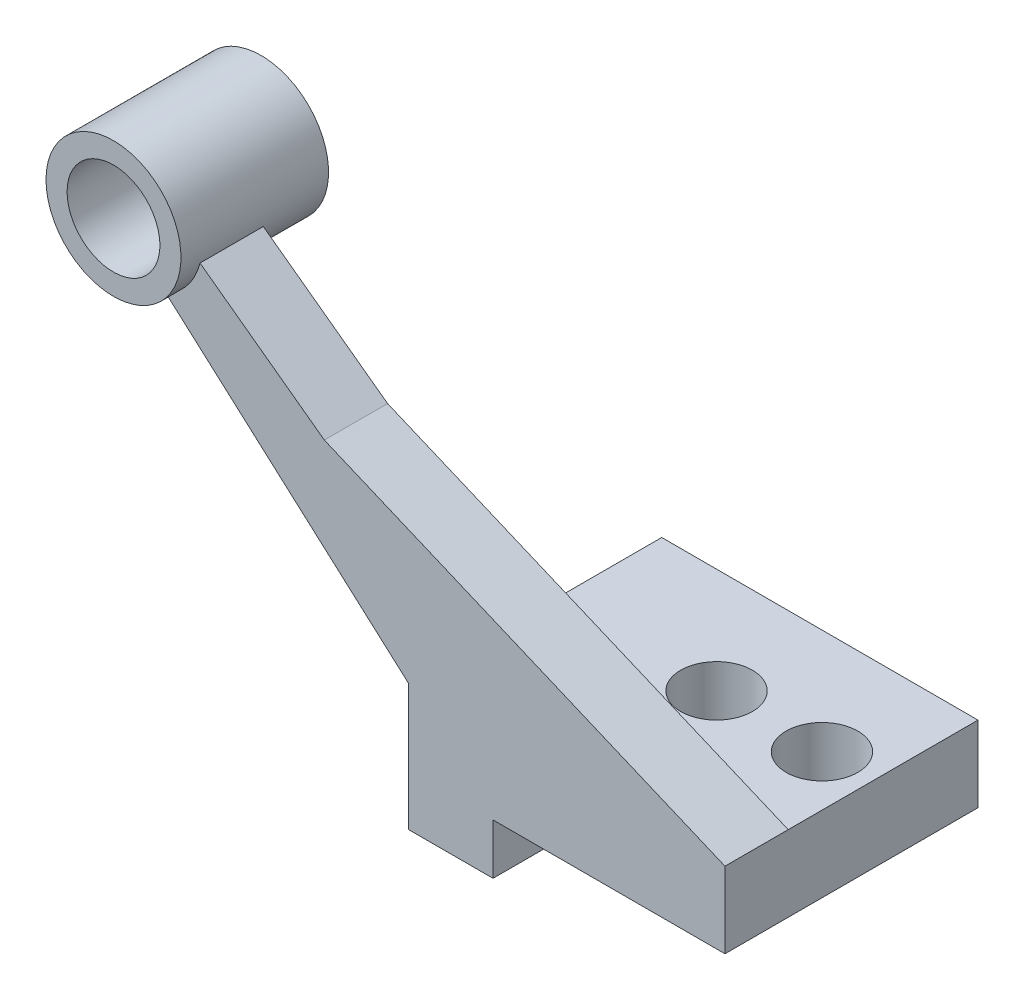
ISO-10303-21;
HEADER;
FILE_DESCRIPTION(('STEP AP214'),'2;1');
FILE_NAME('part.step','',(''),(''),'','','');
FILE_SCHEMA(('AUTOMOTIVE_DESIGN { 1 0 10303 214 1 1 1 1 }'));
ENDSEC;
DATA;
#1=APPLICATION_CONTEXT('core data for automotive mechanical design processes');
#2=APPLICATION_PROTOCOL_DEFINITION('international standard','automotive_design',2000,#1);
#3=PRODUCT_CONTEXT('',#1,'mechanical');
#4=PRODUCT('Part','Part','',(#3));
#5=PRODUCT_RELATED_PRODUCT_CATEGORY('part','',(#4));
#6=PRODUCT_DEFINITION_FORMATION('','',#4);
#7=PRODUCT_DEFINITION_CONTEXT('part definition',#1,'design');
#8=PRODUCT_DEFINITION('design','',#6,#7);
#9=PRODUCT_DEFINITION_SHAPE('','',#8);
#10=(LENGTH_UNIT() NAMED_UNIT(*) SI_UNIT(.MILLI.,.METRE.));
#11=(NAMED_UNIT(*) PLANE_ANGLE_UNIT() SI_UNIT($,.RADIAN.));
#12=(NAMED_UNIT(*) SI_UNIT($,.STERADIAN.) SOLID_ANGLE_UNIT());
#13=UNCERTAINTY_MEASURE_WITH_UNIT(LENGTH_MEASURE(1.E-05),#10,'distance_accuracy_value','');
#14=(GEOMETRIC_REPRESENTATION_CONTEXT(3) GLOBAL_UNCERTAINTY_ASSIGNED_CONTEXT((#13)) GLOBAL_UNIT_ASSIGNED_CONTEXT((#10,
#11,#12)) REPRESENTATION_CONTEXT('',''));
#15=CARTESIAN_POINT('',(0.,0.,0.));
#16=DIRECTION('',(0.,0.,1.));
#17=DIRECTION('',(1.,0.,0.));
#18=AXIS2_PLACEMENT_3D('',#15,#16,#17);
#19=CARTESIAN_POINT('',(0.,0.,45.));
#20=DIRECTION('',(0.,0.,-1.));
#21=DIRECTION('',(-1.,0.,0.));
#22=AXIS2_PLACEMENT_3D('',#19,#20,#21);
#23=PLANE('',#22);
#24=DIRECTION('',(-0.746141301283538,0.665787622683772,0.));
#25=VECTOR('',#24,1.);
#26=CARTESIAN_POINT('',(-140.,58.,45.));
#27=LINE('',#26,#25);
#28=CARTESIAN_POINT('',(-75.,0.,45.));
#29=VERTEX_POINT('',#28);
#30=CARTESIAN_POINT('',(-132.541527054624,51.3447472179725,45.));
#31=VERTEX_POINT('',#30);
#32=EDGE_CURVE('E145',#29,#31,#27,.T.);
#33=ORIENTED_EDGE('',*,*,#32,.T.);
#34=CARTESIAN_POINT('',(-140.,65.5,45.));
#35=DIRECTION('',(0.,0.,-1.));
#36=DIRECTION('',(-1.,0.,0.));
#37=AXIS2_PLACEMENT_3D('',#34,#35,#36);
#38=CIRCLE('',#37,16.);
#39=CARTESIAN_POINT('',(-124.478234627449,61.617372060129,45.));
#40=VERTEX_POINT('',#39);
#41=EDGE_CURVE('E126',#40,#31,#38,.T.);
#42=ORIENTED_EDGE('',*,*,#41,.F.);
#43=DIRECTION('',(0.806404995855705,-0.591363663627518,0.));
#44=VECTOR('',#43,1.);
#45=CARTESIAN_POINT('',(-95.,40.,45.));
#46=LINE('',#45,#44);
#47=CARTESIAN_POINT('',(-95.,40.,45.));
#48=VERTEX_POINT('',#47);
#49=EDGE_CURVE('E133',#40,#48,#46,.T.);
#50=ORIENTED_EDGE('',*,*,#49,.T.);
#51=DIRECTION('',(0.921635375138065,-0.388057000058133,0.));
#52=VECTOR('',#51,1.);
#53=CARTESIAN_POINT('',(0.,0.,45.));
#54=LINE('',#53,#52);
#55=CARTESIAN_POINT('',(0.,0.,45.));
#56=VERTEX_POINT('',#55);
#57=EDGE_CURVE('E142',#48,#56,#54,.T.);
#58=ORIENTED_EDGE('',*,*,#57,.T.);
#59=DIRECTION('',(-1.,0.,0.));
#60=VECTOR('',#59,1.);
#61=CARTESIAN_POINT('',(-75.,0.,45.));
#62=LINE('',#61,#60);
#63=EDGE_CURVE('E159',#56,#29,#62,.T.);
#64=ORIENTED_EDGE('',*,*,#63,.T.);
#65=EDGE_LOOP('',(#33,#42,#50,#58,#64));
#66=FACE_BOUND('',#65,.T.);
#67=ADVANCED_FACE('F44',(#66),#23,.T.);
#68=CARTESIAN_POINT('',(-140.,73.,60.));
#69=DIRECTION('',(0.591363663627518,0.806404995855705,0.));
#70=DIRECTION('',(-0.806404995855705,0.591363663627518,0.));
#71=AXIS2_PLACEMENT_3D('',#68,#69,#70);
#72=PLANE('',#71);
#73=DIRECTION('',(0.,0.,-1.));
#74=VECTOR('',#73,1.);
#75=CARTESIAN_POINT('',(-124.478234627449,61.617372060129,65.));
#76=LINE('',#75,#74);
#77=CARTESIAN_POINT('',(-124.478234627449,61.617372060129,60.));
#78=VERTEX_POINT('',#77);
#79=EDGE_CURVE('E121',#78,#40,#76,.T.);
#80=ORIENTED_EDGE('',*,*,#79,.F.);
#81=DIRECTION('',(0.806404995855705,-0.591363663627518,0.));
#82=VECTOR('',#81,1.);
#83=CARTESIAN_POINT('',(-140.,73.,60.));
#84=LINE('',#83,#82);
#85=CARTESIAN_POINT('',(-95.,40.,60.));
#86=VERTEX_POINT('',#85);
#87=EDGE_CURVE('E170',#78,#86,#84,.T.);
#88=ORIENTED_EDGE('',*,*,#87,.T.);
#89=DIRECTION('',(0.,0.,-1.));
#90=VECTOR('',#89,1.);
#91=CARTESIAN_POINT('',(-95.,40.,60.));
#92=LINE('',#91,#90);
#93=EDGE_CURVE('E140',#86,#48,#92,.T.);
#94=ORIENTED_EDGE('',*,*,#93,.T.);
#95=ORIENTED_EDGE('',*,*,#49,.F.);
#96=EDGE_LOOP('',(#80,#88,#94,#95));
#97=FACE_BOUND('',#96,.T.);
#98=ADVANCED_FACE('F135',(#97),#72,.T.);
#99=CARTESIAN_POINT('',(-75.,0.,60.));
#100=DIRECTION('',(-0.665787622683772,-0.746141301283538,0.));
#101=DIRECTION('',(0.746141301283538,-0.665787622683772,0.));
#102=AXIS2_PLACEMENT_3D('',#99,#100,#101);
#103=PLANE('',#102);
#104=DIRECTION('',(0.,0.,-1.));
#105=VECTOR('',#104,1.);
#106=CARTESIAN_POINT('',(-132.541527054624,51.3447472179725,65.));
#107=LINE('',#106,#105);
#108=CARTESIAN_POINT('',(-132.541527054624,51.3447472179725,60.));
#109=VERTEX_POINT('',#108);
#110=EDGE_CURVE('E67',#31,#109,#107,.F.);
#111=ORIENTED_EDGE('',*,*,#110,.F.);
#112=ORIENTED_EDGE('',*,*,#32,.F.);
#113=DIRECTION('',(0.,0.,-1.));
#114=VECTOR('',#113,1.);
#115=CARTESIAN_POINT('',(-75.,0.,60.));
#116=LINE('',#115,#114);
#117=CARTESIAN_POINT('',(-75.,0.,60.));
#118=VERTEX_POINT('',#117);
#119=EDGE_CURVE('E52',#118,#29,#116,.T.);
#120=ORIENTED_EDGE('',*,*,#119,.F.);
#121=DIRECTION('',(-0.746141301283538,0.665787622683772,0.));
#122=VECTOR('',#121,1.);
#123=CARTESIAN_POINT('',(-75.,0.,60.));
#124=LINE('',#123,#122);
#125=EDGE_CURVE('E172',#118,#109,#124,.T.);
#126=ORIENTED_EDGE('',*,*,#125,.T.);
#127=EDGE_LOOP('',(#111,#112,#120,#126));
#128=FACE_BOUND('',#127,.T.);
#129=ADVANCED_FACE('F213',(#128),#103,.T.);
#130=CARTESIAN_POINT('',(0.,0.,60.));
#131=DIRECTION('',(0.388057000058133,0.921635375138065,0.));
#132=DIRECTION('',(-0.921635375138065,0.388057000058133,0.));
#133=AXIS2_PLACEMENT_3D('',#130,#131,#132);
#134=PLANE('',#133);
#135=DIRECTION('',(0.,0.,-1.));
#136=VECTOR('',#135,1.);
#137=CARTESIAN_POINT('',(0.,0.,60.));
#138=LINE('',#137,#136);
#139=CARTESIAN_POINT('',(0.,0.,60.));
#140=VERTEX_POINT('',#139);
#141=EDGE_CURVE('E11',#140,#56,#138,.T.);
#142=ORIENTED_EDGE('',*,*,#141,.T.);
#143=ORIENTED_EDGE('',*,*,#57,.F.);
#144=ORIENTED_EDGE('',*,*,#93,.F.);
#145=DIRECTION('',(0.921635375138065,-0.388057000058133,0.));
#146=VECTOR('',#145,1.);
#147=CARTESIAN_POINT('',(0.,0.,60.));
#148=LINE('',#147,#146);
#149=EDGE_CURVE('E171',#86,#140,#148,.T.);
#150=ORIENTED_EDGE('',*,*,#149,.T.);
#151=EDGE_LOOP('',(#142,#143,#144,#150));
#152=FACE_BOUND('',#151,.T.);
#153=ADVANCED_FACE('F237',(#152),#134,.T.);
#154=CARTESIAN_POINT('',(0.,-18.,60.));
#155=DIRECTION('',(-1.,0.,0.));
#156=DIRECTION('',(0.,0.,1.));
#157=AXIS2_PLACEMENT_3D('',#154,#155,#156);
#158=PLANE('',#157);
#159=DIRECTION('',(0.,1.,0.));
#160=VECTOR('',#159,1.);
#161=CARTESIAN_POINT('',(0.,-18.,0.));
#162=LINE('',#161,#160);
#163=CARTESIAN_POINT('',(0.,-18.,0.));
#164=VERTEX_POINT('',#163);
#165=CARTESIAN_POINT('',(0.,0.,0.));
#166=VERTEX_POINT('',#165);
#167=EDGE_CURVE('E180',#164,#166,#162,.T.);
#168=ORIENTED_EDGE('',*,*,#167,.T.);
#169=DIRECTION('',(0.,0.,-1.));
#170=VECTOR('',#169,1.);
#171=CARTESIAN_POINT('',(0.,0.,45.));
#172=LINE('',#171,#170);
#173=EDGE_CURVE('E164',#56,#166,#172,.T.);
#174=ORIENTED_EDGE('',*,*,#173,.F.);
#175=ORIENTED_EDGE('',*,*,#141,.F.);
#176=DIRECTION('',(0.,1.,0.));
#177=VECTOR('',#176,1.);
#178=CARTESIAN_POINT('',(0.,-18.,60.));
#179=LINE('',#178,#177);
#180=CARTESIAN_POINT('',(0.,-18.,60.));
#181=VERTEX_POINT('',#180);
#182=EDGE_CURVE('E178',#181,#140,#179,.T.);
#183=ORIENTED_EDGE('',*,*,#182,.F.);
#184=DIRECTION('',(0.,0.,-1.));
#185=VECTOR('',#184,1.);
#186=CARTESIAN_POINT('',(0.,-18.,60.));
#187=LINE('',#186,#185);
#188=EDGE_CURVE('E186',#181,#164,#187,.T.);
#189=ORIENTED_EDGE('',*,*,#188,.T.);
#190=EDGE_LOOP('',(#168,#174,#175,#183,#189));
#191=FACE_BOUND('',#190,.T.);
#192=ADVANCED_FACE('F50',(#191),#158,.F.);
#193=CARTESIAN_POINT('',(-75.,0.,60.));
#194=DIRECTION('',(1.,0.,0.));
#195=DIRECTION('',(0.,0.,-1.));
#196=AXIS2_PLACEMENT_3D('',#193,#194,#195);
#197=PLANE('',#196);
#198=DIRECTION('',(0.,-1.,0.));
#199=VECTOR('',#198,1.);
#200=CARTESIAN_POINT('',(-75.,0.,0.));
#201=LINE('',#200,#199);
#202=CARTESIAN_POINT('',(-75.,0.,0.));
#203=VERTEX_POINT('',#202);
#204=CARTESIAN_POINT('',(-75.,-30.,0.));
#205=VERTEX_POINT('',#204);
#206=EDGE_CURVE('E195',#203,#205,#201,.T.);
#207=ORIENTED_EDGE('',*,*,#206,.T.);
#208=DIRECTION('',(0.,0.,-1.));
#209=VECTOR('',#208,1.);
#210=CARTESIAN_POINT('',(-75.,-30.,60.));
#211=LINE('',#210,#209);
#212=CARTESIAN_POINT('',(-75.,-30.,60.));
#213=VERTEX_POINT('',#212);
#214=EDGE_CURVE('E210',#213,#205,#211,.T.);
#215=ORIENTED_EDGE('',*,*,#214,.F.);
#216=DIRECTION('',(0.,-1.,0.));
#217=VECTOR('',#216,1.);
#218=CARTESIAN_POINT('',(-75.,0.,60.));
#219=LINE('',#218,#217);
#220=EDGE_CURVE('E179',#118,#213,#219,.T.);
#221=ORIENTED_EDGE('',*,*,#220,.F.);
#222=ORIENTED_EDGE('',*,*,#119,.T.);
#223=DIRECTION('',(0.,0.,-1.));
#224=VECTOR('',#223,1.);
#225=CARTESIAN_POINT('',(-75.,0.,45.));
#226=LINE('',#225,#224);
#227=EDGE_CURVE('E161',#29,#203,#226,.T.);
#228=ORIENTED_EDGE('',*,*,#227,.T.);
#229=EDGE_LOOP('',(#207,#215,#221,#222,#228));
#230=FACE_BOUND('',#229,.T.);
#231=ADVANCED_FACE('F215',(#230),#197,.F.);
#232=CARTESIAN_POINT('',(-75.,-30.,60.));
#233=DIRECTION('',(0.,1.,0.));
#234=DIRECTION('',(0.,0.,1.));
#235=AXIS2_PLACEMENT_3D('',#232,#233,#234);
#236=PLANE('',#235);
#237=DIRECTION('',(1.,0.,0.));
#238=VECTOR('',#237,1.);
#239=CARTESIAN_POINT('',(-75.,-30.,0.));
#240=LINE('',#239,#238);
#241=CARTESIAN_POINT('',(-55.,-30.,0.));
#242=VERTEX_POINT('',#241);
#243=EDGE_CURVE('E191',#205,#242,#240,.T.);
#244=ORIENTED_EDGE('',*,*,#243,.T.);
#245=DIRECTION('',(0.,0.,-1.));
#246=VECTOR('',#245,1.);
#247=CARTESIAN_POINT('',(-55.,-30.,60.));
#248=LINE('',#247,#246);
#249=CARTESIAN_POINT('',(-55.,-30.,60.));
#250=VERTEX_POINT('',#249);
#251=EDGE_CURVE('E204',#250,#242,#248,.T.);
#252=ORIENTED_EDGE('',*,*,#251,.F.);
#253=DIRECTION('',(1.,0.,0.));
#254=VECTOR('',#253,1.);
#255=CARTESIAN_POINT('',(-75.,-30.,60.));
#256=LINE('',#255,#254);
#257=EDGE_CURVE('E182',#213,#250,#256,.T.);
#258=ORIENTED_EDGE('',*,*,#257,.F.);
#259=ORIENTED_EDGE('',*,*,#214,.T.);
#260=EDGE_LOOP('',(#244,#252,#258,#259));
#261=FACE_BOUND('',#260,.T.);
#262=ADVANCED_FACE('F223',(#261),#236,.F.);
#263=CARTESIAN_POINT('',(-55.,-30.,60.));
#264=DIRECTION('',(-1.,0.,0.));
#265=DIRECTION('',(0.,0.,1.));
#266=AXIS2_PLACEMENT_3D('',#263,#264,#265);
#267=PLANE('',#266);
#268=DIRECTION('',(0.,1.,0.));
#269=VECTOR('',#268,1.);
#270=CARTESIAN_POINT('',(-55.,-30.,0.));
#271=LINE('',#270,#269);
#272=CARTESIAN_POINT('',(-55.,-18.,0.));
#273=VERTEX_POINT('',#272);
#274=EDGE_CURVE('E196',#242,#273,#271,.T.);
#275=ORIENTED_EDGE('',*,*,#274,.T.);
#276=DIRECTION('',(0.,0.,-1.));
#277=VECTOR('',#276,1.);
#278=CARTESIAN_POINT('',(-55.,-18.,60.));
#279=LINE('',#278,#277);
#280=CARTESIAN_POINT('',(-55.,-18.,60.));
#281=VERTEX_POINT('',#280);
#282=EDGE_CURVE('E203',#281,#273,#279,.T.);
#283=ORIENTED_EDGE('',*,*,#282,.F.);
#284=DIRECTION('',(0.,1.,0.));
#285=VECTOR('',#284,1.);
#286=CARTESIAN_POINT('',(-55.,-30.,60.));
#287=LINE('',#286,#285);
#288=EDGE_CURVE('E184',#250,#281,#287,.T.);
#289=ORIENTED_EDGE('',*,*,#288,.F.);
#290=ORIENTED_EDGE('',*,*,#251,.T.);
#291=EDGE_LOOP('',(#275,#283,#289,#290));
#292=FACE_BOUND('',#291,.T.);
#293=ADVANCED_FACE('F228',(#292),#267,.F.);
#294=CARTESIAN_POINT('',(-55.,-18.,60.));
#295=DIRECTION('',(0.,1.,0.));
#296=DIRECTION('',(0.,0.,1.));
#297=AXIS2_PLACEMENT_3D('',#294,#295,#296);
#298=PLANE('',#297);
#299=CARTESIAN_POINT('',(-12.,-18.,25.));
#300=DIRECTION('',(0.,1.,0.));
#301=DIRECTION('',(0.,0.,1.));
#302=AXIS2_PLACEMENT_3D('',#299,#300,#301);
#303=CIRCLE('',#302,8.5);
#304=CARTESIAN_POINT('',(-12.,-18.,33.5));
#305=VERTEX_POINT('',#304);
#306=EDGE_CURVE('E287',#305,#305,#303,.T.);
#307=ORIENTED_EDGE('',*,*,#306,.T.);
#308=EDGE_LOOP('',(#307));
#309=FACE_BOUND('',#308,.T.);
#310=CARTESIAN_POINT('',(-37.,-18.,25.));
#311=DIRECTION('',(0.,1.,0.));
#312=DIRECTION('',(0.,0.,1.));
#313=AXIS2_PLACEMENT_3D('',#310,#311,#312);
#314=CIRCLE('',#313,8.5);
#315=CARTESIAN_POINT('',(-37.,-18.,33.5));
#316=VERTEX_POINT('',#315);
#317=EDGE_CURVE('E291',#316,#316,#314,.T.);
#318=ORIENTED_EDGE('',*,*,#317,.T.);
#319=EDGE_LOOP('',(#318));
#320=FACE_BOUND('',#319,.T.);
#321=DIRECTION('',(1.,0.,0.));
#322=VECTOR('',#321,1.);
#323=CARTESIAN_POINT('',(-55.,-18.,0.));
#324=LINE('',#323,#322);
#325=EDGE_CURVE('E181',#273,#164,#324,.T.);
#326=ORIENTED_EDGE('',*,*,#325,.T.);
#327=ORIENTED_EDGE('',*,*,#188,.F.);
#328=DIRECTION('',(1.,0.,0.));
#329=VECTOR('',#328,1.);
#330=CARTESIAN_POINT('',(-55.,-18.,60.));
#331=LINE('',#330,#329);
#332=EDGE_CURVE('E190',#281,#181,#331,.T.);
#333=ORIENTED_EDGE('',*,*,#332,.F.);
#334=ORIENTED_EDGE('',*,*,#282,.T.);
#335=EDGE_LOOP('',(#326,#327,#333,#334));
#336=FACE_BOUND('',#335,.T.);
#337=ADVANCED_FACE('F231',(#309,#320,#336),#298,.F.);
#338=CARTESIAN_POINT('',(0.,0.,60.));
#339=DIRECTION('',(0.,0.,1.));
#340=DIRECTION('',(1.,0.,0.));
#341=AXIS2_PLACEMENT_3D('',#338,#339,#340);
#342=PLANE('',#341);
#343=CARTESIAN_POINT('',(-140.,65.5,60.));
#344=DIRECTION('',(0.,0.,1.));
#345=DIRECTION('',(1.,0.,0.));
#346=AXIS2_PLACEMENT_3D('',#343,#344,#345);
#347=CIRCLE('',#346,16.);
#348=EDGE_CURVE('E58',#109,#78,#347,.T.);
#349=ORIENTED_EDGE('',*,*,#348,.F.);
#350=ORIENTED_EDGE('',*,*,#125,.F.);
#351=ORIENTED_EDGE('',*,*,#220,.T.);
#352=ORIENTED_EDGE('',*,*,#257,.T.);
#353=ORIENTED_EDGE('',*,*,#288,.T.);
#354=ORIENTED_EDGE('',*,*,#332,.T.);
#355=ORIENTED_EDGE('',*,*,#182,.T.);
#356=ORIENTED_EDGE('',*,*,#149,.F.);
#357=ORIENTED_EDGE('',*,*,#87,.F.);
#358=EDGE_LOOP('',(#349,#350,#351,#352,#353,#354,#355,#356,#357));
#359=FACE_BOUND('',#358,.T.);
#360=ADVANCED_FACE('F216',(#359),#342,.T.);
#361=CARTESIAN_POINT('',(0.,0.,0.));
#362=DIRECTION('',(0.,0.,1.));
#363=DIRECTION('',(1.,0.,0.));
#364=AXIS2_PLACEMENT_3D('',#361,#362,#363);
#365=PLANE('',#364);
#366=ORIENTED_EDGE('',*,*,#206,.F.);
#367=DIRECTION('',(-1.,0.,0.));
#368=VECTOR('',#367,1.);
#369=CARTESIAN_POINT('',(-75.,0.,0.));
#370=LINE('',#369,#368);
#371=EDGE_CURVE('E131',#166,#203,#370,.T.);
#372=ORIENTED_EDGE('',*,*,#371,.F.);
#373=ORIENTED_EDGE('',*,*,#167,.F.);
#374=ORIENTED_EDGE('',*,*,#325,.F.);
#375=ORIENTED_EDGE('',*,*,#274,.F.);
#376=ORIENTED_EDGE('',*,*,#243,.F.);
#377=EDGE_LOOP('',(#366,#372,#373,#374,#375,#376));
#378=FACE_BOUND('',#377,.T.);
#379=ADVANCED_FACE('F242',(#378),#365,.F.);
#380=CARTESIAN_POINT('',(-75.,0.,45.));
#381=DIRECTION('',(0.,-1.,0.));
#382=DIRECTION('',(0.,0.,-1.));
#383=AXIS2_PLACEMENT_3D('',#380,#381,#382);
#384=PLANE('',#383);
#385=CARTESIAN_POINT('',(-12.,0.,25.));
#386=DIRECTION('',(0.,1.,0.));
#387=DIRECTION('',(0.,0.,1.));
#388=AXIS2_PLACEMENT_3D('',#385,#386,#387);
#389=CIRCLE('',#388,8.5);
#390=CARTESIAN_POINT('',(-12.,0.,33.5));
#391=VERTEX_POINT('',#390);
#392=EDGE_CURVE('E294',#391,#391,#389,.T.);
#393=ORIENTED_EDGE('',*,*,#392,.F.);
#394=EDGE_LOOP('',(#393));
#395=FACE_BOUND('',#394,.T.);
#396=CARTESIAN_POINT('',(-37.,0.,25.));
#397=DIRECTION('',(0.,1.,0.));
#398=DIRECTION('',(0.,0.,1.));
#399=AXIS2_PLACEMENT_3D('',#396,#397,#398);
#400=CIRCLE('',#399,8.5);
#401=CARTESIAN_POINT('',(-37.,0.,33.5));
#402=VERTEX_POINT('',#401);
#403=EDGE_CURVE('E298',#402,#402,#400,.T.);
#404=ORIENTED_EDGE('',*,*,#403,.F.);
#405=EDGE_LOOP('',(#404));
#406=FACE_BOUND('',#405,.T.);
#407=ORIENTED_EDGE('',*,*,#371,.T.);
#408=ORIENTED_EDGE('',*,*,#227,.F.);
#409=ORIENTED_EDGE('',*,*,#63,.F.);
#410=ORIENTED_EDGE('',*,*,#173,.T.);
#411=EDGE_LOOP('',(#407,#408,#409,#410));
#412=FACE_BOUND('',#411,.T.);
#413=ADVANCED_FACE('F241',(#395,#406,#412),#384,.F.);
#414=CARTESIAN_POINT('',(-140.,65.5,65.));
#415=DIRECTION('',(0.,0.,-1.));
#416=DIRECTION('',(-1.,0.,0.));
#417=AXIS2_PLACEMENT_3D('',#414,#415,#416);
#418=CYLINDRICAL_SURFACE('',#417,16.);
#419=CARTESIAN_POINT('',(-140.,65.5,65.));
#420=DIRECTION('',(0.,0.,-1.));
#421=DIRECTION('',(-1.,0.,0.));
#422=AXIS2_PLACEMENT_3D('',#419,#420,#421);
#423=CIRCLE('',#422,16.);
#424=CARTESIAN_POINT('',(-156.,65.5,65.));
#425=VERTEX_POINT('',#424);
#426=EDGE_CURVE('E146',#425,#425,#423,.T.);
#427=ORIENTED_EDGE('',*,*,#426,.T.);
#428=EDGE_LOOP('',(#427));
#429=FACE_BOUND('',#428,.T.);
#430=ORIENTED_EDGE('',*,*,#348,.T.);
#431=ORIENTED_EDGE('',*,*,#79,.T.);
#432=ORIENTED_EDGE('',*,*,#41,.T.);
#433=ORIENTED_EDGE('',*,*,#110,.T.);
#434=EDGE_LOOP('',(#430,#431,#432,#433));
#435=FACE_BOUND('',#434,.T.);
#436=CARTESIAN_POINT('',(-140.,65.5,30.));
#437=DIRECTION('',(0.,0.,-1.));
#438=DIRECTION('',(-1.,0.,0.));
#439=AXIS2_PLACEMENT_3D('',#436,#437,#438);
#440=CIRCLE('',#439,16.);
#441=CARTESIAN_POINT('',(-156.,65.5,30.));
#442=VERTEX_POINT('',#441);
#443=EDGE_CURVE('E143',#442,#442,#440,.T.);
#444=ORIENTED_EDGE('',*,*,#443,.F.);
#445=EDGE_LOOP('',(#444));
#446=FACE_BOUND('',#445,.T.);
#447=ADVANCED_FACE('F127',(#429,#435,#446),#418,.T.);
#448=CARTESIAN_POINT('',(-140.,65.5,65.));
#449=DIRECTION('',(0.,0.,-1.));
#450=DIRECTION('',(-1.,0.,0.));
#451=AXIS2_PLACEMENT_3D('',#448,#449,#450);
#452=PLANE('',#451);
#453=CARTESIAN_POINT('',(-140.,65.5,65.));
#454=DIRECTION('',(0.,0.,-1.));
#455=DIRECTION('',(-1.,0.,0.));
#456=AXIS2_PLACEMENT_3D('',#453,#454,#455);
#457=CIRCLE('',#456,11.);
#458=CARTESIAN_POINT('',(-151.,65.5,65.));
#459=VERTEX_POINT('',#458);
#460=EDGE_CURVE('E147',#459,#459,#457,.T.);
#461=ORIENTED_EDGE('',*,*,#460,.T.);
#462=EDGE_LOOP('',(#461));
#463=FACE_BOUND('',#462,.T.);
#464=ORIENTED_EDGE('',*,*,#426,.F.);
#465=EDGE_LOOP('',(#464));
#466=FACE_BOUND('',#465,.T.);
#467=ADVANCED_FACE('F312',(#463,#466),#452,.F.);
#468=CARTESIAN_POINT('',(-140.,65.5,30.));
#469=DIRECTION('',(0.,0.,-1.));
#470=DIRECTION('',(-1.,0.,0.));
#471=AXIS2_PLACEMENT_3D('',#468,#469,#470);
#472=PLANE('',#471);
#473=CARTESIAN_POINT('',(-140.,65.5,30.));
#474=DIRECTION('',(0.,0.,-1.));
#475=DIRECTION('',(-1.,0.,0.));
#476=AXIS2_PLACEMENT_3D('',#473,#474,#475);
#477=CIRCLE('',#476,11.);
#478=CARTESIAN_POINT('',(-151.,65.5,30.));
#479=VERTEX_POINT('',#478);
#480=EDGE_CURVE('E152',#479,#479,#477,.T.);
#481=ORIENTED_EDGE('',*,*,#480,.F.);
#482=EDGE_LOOP('',(#481));
#483=FACE_BOUND('',#482,.T.);
#484=ORIENTED_EDGE('',*,*,#443,.T.);
#485=EDGE_LOOP('',(#484));
#486=FACE_BOUND('',#485,.T.);
#487=ADVANCED_FACE('F309',(#483,#486),#472,.T.);
#488=CARTESIAN_POINT('',(-140.,65.5,70.));
#489=DIRECTION('',(0.,0.,-1.));
#490=DIRECTION('',(-1.,0.,0.));
#491=AXIS2_PLACEMENT_3D('',#488,#489,#490);
#492=CYLINDRICAL_SURFACE('',#491,11.);
#493=ORIENTED_EDGE('',*,*,#480,.T.);
#494=EDGE_LOOP('',(#493));
#495=FACE_BOUND('',#494,.T.);
#496=ORIENTED_EDGE('',*,*,#460,.F.);
#497=EDGE_LOOP('',(#496));
#498=FACE_BOUND('',#497,.T.);
#499=ADVANCED_FACE('F310',(#495,#498),#492,.F.);
#500=CARTESIAN_POINT('',(-37.,-18.,25.));
#501=DIRECTION('',(0.,1.,0.));
#502=DIRECTION('',(0.,0.,1.));
#503=AXIS2_PLACEMENT_3D('',#500,#501,#502);
#504=CYLINDRICAL_SURFACE('',#503,8.5);
#505=ORIENTED_EDGE('',*,*,#317,.F.);
#506=EDGE_LOOP('',(#505));
#507=FACE_BOUND('',#506,.T.);
#508=ORIENTED_EDGE('',*,*,#403,.T.);
#509=EDGE_LOOP('',(#508));
#510=FACE_BOUND('',#509,.T.);
#511=ADVANCED_FACE('F329',(#507,#510),#504,.F.);
#512=CARTESIAN_POINT('',(-12.,-18.,25.));
#513=DIRECTION('',(0.,1.,0.));
#514=DIRECTION('',(0.,0.,1.));
#515=AXIS2_PLACEMENT_3D('',#512,#513,#514);
#516=CYLINDRICAL_SURFACE('',#515,8.5);
#517=ORIENTED_EDGE('',*,*,#306,.F.);
#518=EDGE_LOOP('',(#517));
#519=FACE_BOUND('',#518,.T.);
#520=ORIENTED_EDGE('',*,*,#392,.T.);
#521=EDGE_LOOP('',(#520));
#522=FACE_BOUND('',#521,.T.);
#523=ADVANCED_FACE('F333',(#519,#522),#516,.F.);
#524=CLOSED_SHELL('',(#67,#98,#129,#153,#192,#231,#262,#293,#337,#360,#379,#413,#447,#467,#487,
#499,#511,#523));
#525=MANIFOLD_SOLID_BREP('B2',#524);
#526=ADVANCED_BREP_SHAPE_REPRESENTATION('',(#18,#525),#14);
#527=SHAPE_DEFINITION_REPRESENTATION(#9,#526);
ENDSEC;
END-ISO-10303-21;
